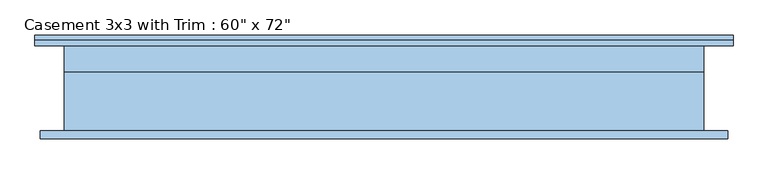
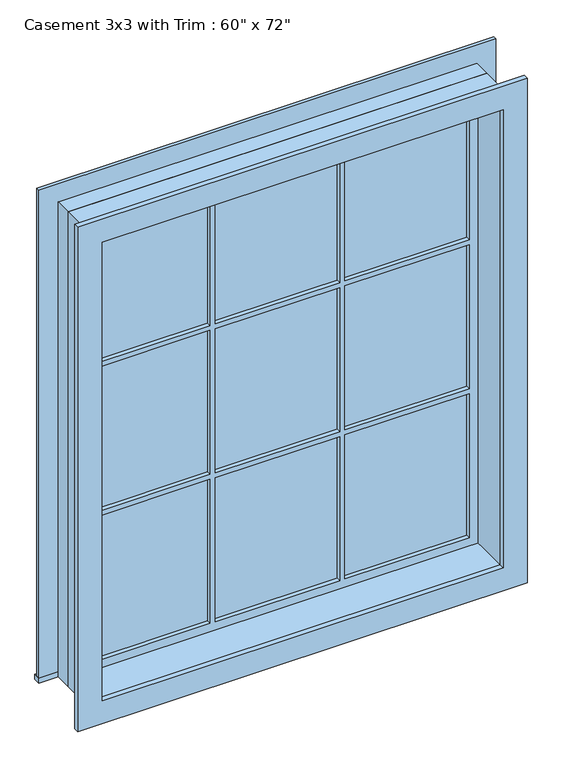
"""IFC4 building model written with IfcOpenShell, lengths in millimetres: window geometry."""

from ifc_helpers import new_model, si_unit, frame, origin, place, context, project, spatial, polyline, outline, extrude, source, transform, mapped, element, save


def window_cc15f82e(model_context):
    return source(origin(), model_context, "Body", "SweptSolid", [
        extrude(outline(polyline([(-831.85, 127.0), (831.85, 127.0), (831.85, 101.6), (-831.85, 101.6), (-831.85, 127.0)])), frame((0.0, 0.0, 304.8), z_axis=(0.0, 0.0, 1.0), x_axis=(1.0, 0.0, 0.0)), (0.0, 0.0, 1.0), 19.05),
        extrude(outline(polyline([(2114.55, -742.95), (2114.55, 742.95), (323.85, 742.95), (323.85, 831.85), (2203.45, 831.85), (2203.45, -831.85), (323.85, -831.85), (323.85, -742.95), (2114.55, -742.95)])), frame((0.0, 101.6, 0.0), z_axis=(0.0, 1.0, 0.0), x_axis=(0.0, 0.0, 1.0)), (0.0, 0.0, 1.0), 12.7),
        extrude(outline(polyline([(245.5333333, 66.675), (698.5, 66.675), (698.5, 53.975), (245.5333333, 53.975), (245.5333333, 66.675)])), frame((0.0, 0.0, 1515.5333333), z_axis=(0.0, 0.0, 1.0), x_axis=(1.0, 0.0, 0.0)), (0.0, 0.0, 1.0), 554.5666667),
        extrude(outline(polyline([(-226.4833333, 66.675), (226.4833333, 66.675), (226.4833333, 53.975), (-226.4833333, 53.975), (-226.4833333, 66.675)])), frame((0.0, 0.0, 1515.5333333), z_axis=(0.0, 0.0, 1.0), x_axis=(1.0, 0.0, 0.0)), (0.0, 0.0, 1.0), 554.5666667),
        extrude(outline(polyline([(-698.5, 66.675), (-245.5333333, 66.675), (-245.5333333, 53.975), (-698.5, 53.975), (-698.5, 66.675)])), frame((0.0, 0.0, 1515.5333333), z_axis=(0.0, 0.0, 1.0), x_axis=(1.0, 0.0, 0.0)), (0.0, 0.0, 1.0), 554.5666667),
        extrude(outline(polyline([(-698.5, 66.675), (-245.5333333, 66.675), (-245.5333333, 53.975), (-698.5, 53.975), (-698.5, 66.675)])), frame((0.0, 0.0, 941.9166667), z_axis=(0.0, 0.0, 1.0), x_axis=(1.0, 0.0, 0.0)), (0.0, 0.0, 1.0), 554.5666667),
        extrude(outline(polyline([(-226.4833333, 66.675), (226.4833333, 66.675), (226.4833333, 53.975), (-226.4833333, 53.975), (-226.4833333, 66.675)])), frame((0.0, 0.0, 941.9166667), z_axis=(0.0, 0.0, 1.0), x_axis=(1.0, 0.0, 0.0)), (0.0, 0.0, 1.0), 554.5666667),
        extrude(outline(polyline([(245.5333333, 66.675), (698.5, 66.675), (698.5, 53.975), (245.5333333, 53.975), (245.5333333, 66.675)])), frame((0.0, 0.0, 941.9166667), z_axis=(0.0, 0.0, 1.0), x_axis=(1.0, 0.0, 0.0)), (0.0, 0.0, 1.0), 554.5666667),
        extrude(outline(polyline([(245.5333333, 66.675), (698.5, 66.675), (698.5, 53.975), (245.5333333, 53.975), (245.5333333, 66.675)])), frame((0.0, 0.0, 368.3), z_axis=(0.0, 0.0, 1.0), x_axis=(1.0, 0.0, 0.0)), (0.0, 0.0, 1.0), 554.5666667),
        extrude(outline(polyline([(-226.4833333, 66.675), (226.4833333, 66.675), (226.4833333, 53.975), (-226.4833333, 53.975), (-226.4833333, 66.675)])), frame((0.0, 0.0, 368.3), z_axis=(0.0, 0.0, 1.0), x_axis=(1.0, 0.0, 0.0)), (0.0, 0.0, 1.0), 554.5666667),
        extrude(outline(polyline([(-698.5, 66.675), (-245.5333333, 66.675), (-245.5333333, 53.975), (-698.5, 53.975), (-698.5, 66.675)])), frame((0.0, 0.0, 368.3), z_axis=(0.0, 0.0, 1.0), x_axis=(1.0, 0.0, 0.0)), (0.0, 0.0, 1.0), 554.5666667),
        extrude(outline(polyline([(2190.75, 819.15), (2190.75, -819.15), (247.65, -819.15), (247.65, 819.15), (2190.75, 819.15)]), holes=[polyline([(2101.85, 730.25), (336.55, 730.25), (336.55, -730.25), (2101.85, -730.25), (2101.85, 730.25)])]), frame((0.0, -120.65, 0.0), z_axis=(0.0, 1.0, 0.0), x_axis=(0.0, 0.0, 1.0)), (0.0, 0.0, 1.0), 19.05),
        extrude(outline(polyline([(2114.55, -742.95), (323.85, -742.95), (323.85, 742.95), (2114.55, 742.95), (2114.55, -742.95)]), holes=[polyline([(2070.1, -245.5333333), (1515.5333333, -245.5333333), (1515.5333333, -698.5), (2070.1, -698.5), (2070.1, -245.5333333)]), polyline([(1496.4833333, -245.5333333), (941.9166667, -245.5333333), (941.9166667, -698.5), (1496.4833333, -698.5), (1496.4833333, -245.5333333)]), polyline([(922.8666667, -245.5333333), (368.3, -245.5333333), (368.3, -698.5), (922.8666667, -698.5), (922.8666667, -245.5333333)]), polyline([(2070.1, 226.4833333), (1515.5333333, 226.4833333), (1515.5333333, -226.4833333), (2070.1, -226.4833333), (2070.1, 226.4833333)]), polyline([(1496.4833333, 226.4833333), (941.9166667, 226.4833333), (941.9166667, -226.4833333), (1496.4833333, -226.4833333), (1496.4833333, 226.4833333)]), polyline([(922.8666667, 226.4833333), (368.3, 226.4833333), (368.3, -226.4833333), (922.8666667, -226.4833333), (922.8666667, 226.4833333)]), polyline([(2070.1, 698.5), (1515.5333333, 698.5), (1515.5333333, 245.5333333), (2070.1, 245.5333333), (2070.1, 698.5)]), polyline([(1496.4833333, 698.5), (941.9166667, 698.5), (941.9166667, 245.5333333), (1496.4833333, 245.5333333), (1496.4833333, 698.5)]), polyline([(922.8666667, 698.5), (368.3, 698.5), (368.3, 245.5333333), (922.8666667, 245.5333333), (922.8666667, 698.5)])]), frame((0.0, 38.1, 0.0), z_axis=(0.0, 1.0, 0.0), x_axis=(0.0, 0.0, 1.0)), (0.0, 0.0, 1.0), 44.45),
        extrude(outline(polyline([(2133.6, -762.0), (304.8, -762.0), (304.8, 762.0), (2133.6, 762.0), (2133.6, -762.0)]), holes=[polyline([(2101.85, -730.25), (2101.85, 730.25), (336.55, 730.25), (336.55, -730.25), (2101.85, -730.25)])]), frame((0.0, -101.6, 0.0), z_axis=(0.0, 1.0, 0.0), x_axis=(0.0, 0.0, 1.0)), (0.0, 0.0, 1.0), 139.7),
        extrude(outline(polyline([(2133.6, 762.0), (2133.6, -762.0), (304.8, -762.0), (304.8, 762.0), (2133.6, 762.0)]), holes=[polyline([(2114.55, 742.95), (323.85, 742.95), (323.85, -742.95), (2114.55, -742.95), (2114.55, 742.95)])]), frame((0.0, 38.1, 0.0), z_axis=(0.0, 1.0, 0.0), x_axis=(0.0, 0.0, 1.0)), (0.0, 0.0, 1.0), 63.5),
    ])


if __name__ == "__main__":
    model = new_model("IFC4")
    model_context = context("Model", 3, world=origin())
    ifc_project = project(units=[si_unit("LENGTHUNIT", "METRE", prefix="MILLI")], contexts=[model_context])
    site = spatial("IfcSite", under=ifc_project)
    building = spatial("IfcBuilding", under=site)
    placement = place(None, origin())
    window_shape = window_cc15f82e(model_context)
    element("IfcWindow", 1, ObjectType="Casement 3x3 with Trim : 60\" x 72\"", at=placement, inside=building, context=model_context, shape_type="MappedRepresentation", body=[
        mapped(window_shape, transform((0.0, 0.0, 0.0), x_axis=(1.0, 0.0, 0.0), y_axis=(0.0, 1.0, 0.0), z_axis=(0.0, 0.0, 1.0))),
    ])
    save(model, "model.ifc")

# Revit data of these elements
# Type "Casement 3x3 with Trim : 60\" x 72\""
#   Type Mark = "12"
#   Construction Type Id = "GSP4R"
#   Assembly Code = "B2020100"
#   Analytic Construction = "1/8 in Pilkington single glazing"
#   Visual Light Transmittance = 0.9
#   Solar Heat Gain Coefficient = 0.78
#   Heat Transfer Coefficient (U) = 0.6496 BTU/(h·ft²·°F)
#   Height = 6' - 0"
#   Default Sill Height = 1' - 0"
#   Trim Projection - Ext. = 0' - 0 1/2"
#   Trim Projection - Int. = 0' - 0 3/4"
#   Trim Width - Exterior = 0' - 3 1/2"
#   Trim Width - Interior = 0' - 3 1/2"
#   Width = 5' - 0"
#   Window Inset = 0' - 0 3/4"
#   Define Thermal Properties by = 1
#   Glass Pane Material = Glass
#   Sash Material = Sash
#   Trim Exterior Material = Trim
#   Trim Interior Material = Trim
#   Wall Closure = (empty or 0)
# Element 1 (IfcWindow, "Casement 3x3 with Trim : 60\" x 72\"")
#   Materials on its faces: "Sash", "Glass", "Trim"
# Materials
#   "Glass": class "Glass", colour RGB 0 128 192, transparency 0.75, Description = "Soda Lime Glass", Cost = 0
#   "Sash": class "Wood", colour RGB 224 178 126, transparency 0
#   "Trim": class "Wood", colour RGB 224 178 126, transparency 0
